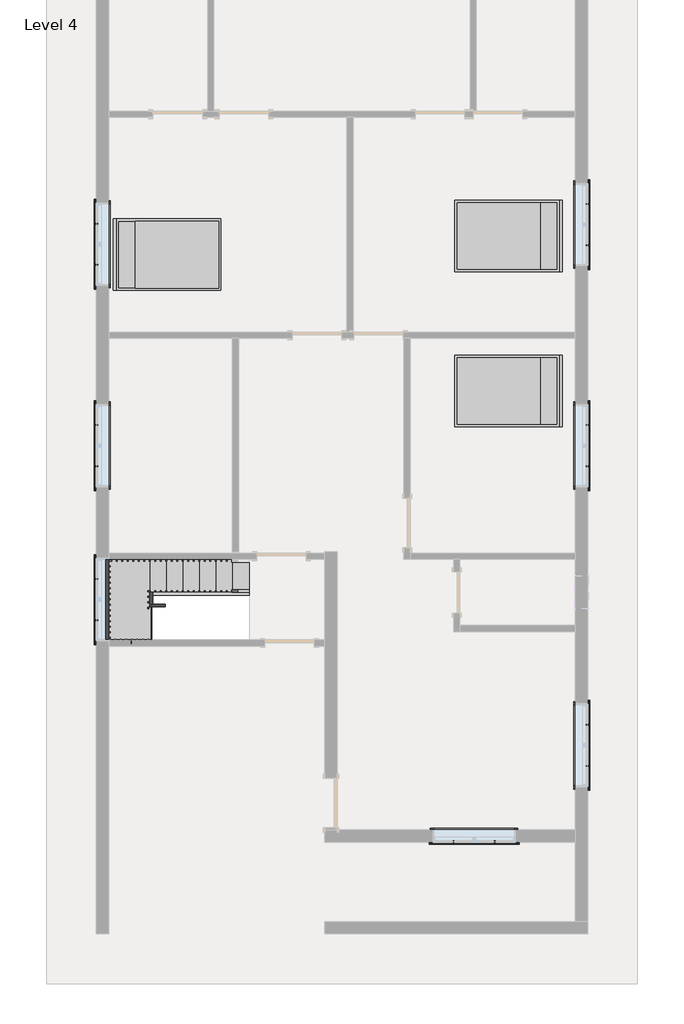
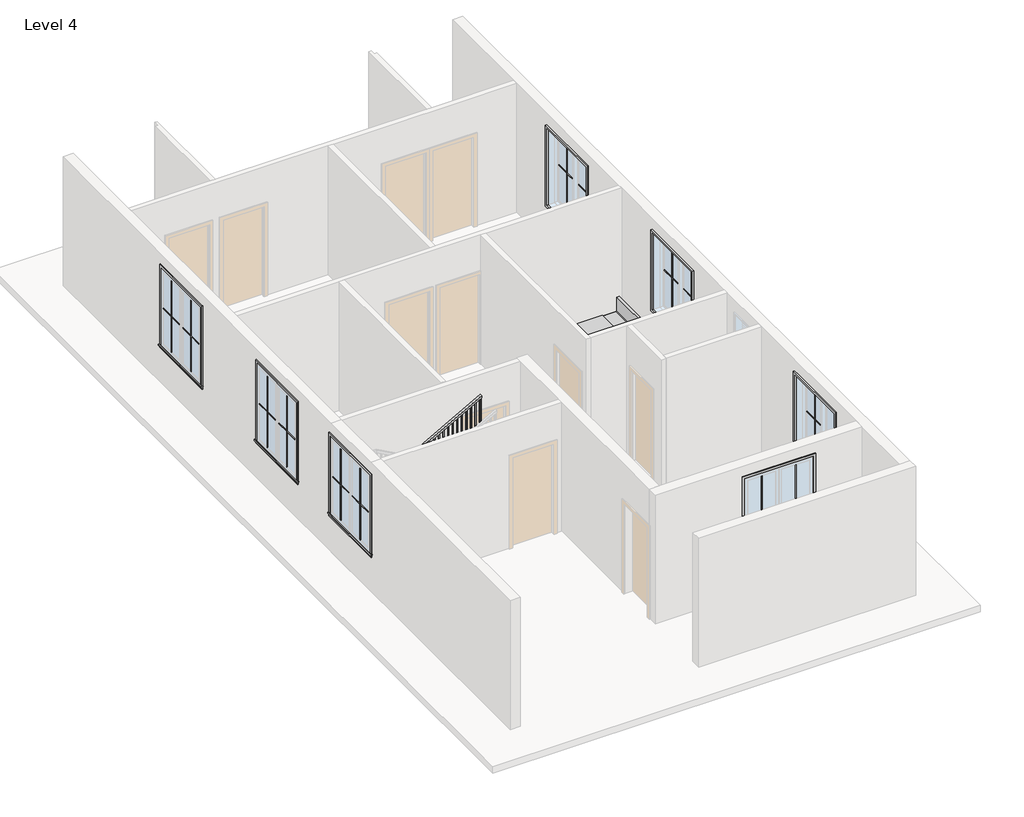
# One storey, part 3 of 3: 28 proxies, 6 members, 3 furniture elements, 1 railing, 1 stair flight.
"""IFC4 building model written with IfcOpenShell, lengths in millimetres."""

from ifc_helpers import new_model, si_unit, frame, origin, place, context, project, spatial, polyline, outline, extrude, faceted_brep, transform, mapped, element, save
from components import muntin_pattern_2x2_muntin_pattern_2x2_f6a80940, muntin_pattern_2x2_muntin_pattern_2x2_09b00a1c, trim_window_exterior_flat_with_sill_698ed857, trim_window_interior_flat_picture_frame_92551a5e, bed_17739_bed_17739_15c61121, stair_flight_6f8696f7

model = new_model("IFC4")

# Units and contexts
model_context = context("Model", 3, world=origin())
ifc_project = project(units=[si_unit("LENGTHUNIT", "METRE", prefix="MILLI")], contexts=[model_context])

# Site, building, storey
site = spatial("IfcSite", under=ifc_project)
building = spatial("IfcBuilding", under=site)
storey = spatial("IfcBuildingStorey", under=building, Name="Level 4", Elevation=6400.8)

# Proxies
placement = place(None, origin())
muntin_pattern_2x2_muntin_pattern_2x2_shape = muntin_pattern_2x2_muntin_pattern_2x2_f6a80940(model_context)
element("IfcBuildingElementProxy", 1, Name="Muntin Pattern_2x2 : Muntin Pattern_2x2", ObjectType="Muntin Pattern_2x2 : Muntin Pattern_2x2", at=placement, inside=storey, context=model_context, shape_type="MappedRepresentation", body=[
    mapped(muntin_pattern_2x2_muntin_pattern_2x2_shape, transform((-5778.6870155, 3260.8309309, 7385.05), x_axis=(0.0, 1.0, 0.0), y_axis=(-1.0, 0.0, 0.0), z_axis=(0.0, 0.0, 1.0))),
])
element("IfcBuildingElementProxy", 2, Name="Muntin Pattern_2x2 : Muntin Pattern_2x2", ObjectType="Muntin Pattern_2x2 : Muntin Pattern_2x2", at=placement, inside=storey, context=model_context, shape_type="MappedRepresentation", body=[
    mapped(muntin_pattern_2x2_muntin_pattern_2x2_shape, transform((3270.0629845, 4381.6059309, 7385.05), x_axis=(0.0, -1.0, 0.0), y_axis=(1.0, 0.0, 0.0), z_axis=(0.0, 0.0, 1.0))),
])
element("IfcBuildingElementProxy", 3, Name="Muntin Pattern_2x2 : Muntin Pattern_2x2", ObjectType="Muntin Pattern_2x2 : Muntin Pattern_2x2", at=placement, inside=storey, context=model_context, shape_type="MappedRepresentation", body=[
    mapped(muntin_pattern_2x2_muntin_pattern_2x2_shape, transform((3270.0629845, 304.9059309, 7385.05), x_axis=(0.0, -1.0, 0.0), y_axis=(1.0, 0.0, 0.0), z_axis=(0.0, 0.0, 1.0))),
])
element("IfcBuildingElementProxy", 4, Name="Muntin Pattern_2x2 : Muntin Pattern_2x2", ObjectType="Muntin Pattern_2x2 : Muntin Pattern_2x2", at=placement, inside=storey, context=model_context, shape_type="MappedRepresentation", body=[
    mapped(muntin_pattern_2x2_muntin_pattern_2x2_shape, transform((3270.0629845, -5219.5940691, 7385.05), x_axis=(0.0, -1.0, 0.0), y_axis=(1.0, 0.0, 0.0), z_axis=(0.0, 0.0, 1.0))),
])
element("IfcBuildingElementProxy", 5, Name="Muntin Pattern_2x2 : Muntin Pattern_2x2", ObjectType="Muntin Pattern_2x2 : Muntin Pattern_2x2", at=placement, inside=storey, context=model_context, shape_type="MappedRepresentation", body=[
    mapped(muntin_pattern_2x2_muntin_pattern_2x2_shape, transform((1563.5004845, -7380.1815691, 7385.05), x_axis=(-1.0, 0.0, 0.0), y_axis=(0.0, -1.0, 0.0), z_axis=(0.0, 0.0, 1.0))),
])
element("IfcBuildingElementProxy", 6, Name="Muntin Pattern_2x2 : Muntin Pattern_2x2", ObjectType="Muntin Pattern_2x2 : Muntin Pattern_2x2", at=placement, inside=storey, context=model_context, shape_type="MappedRepresentation", body=[
    mapped(muntin_pattern_2x2_muntin_pattern_2x2_shape, transform((-5778.6870155, -3292.3690691, 7385.05), x_axis=(0.0, 1.0, 0.0), y_axis=(-1.0, 0.0, 0.0), z_axis=(0.0, 0.0, 1.0))),
])
element("IfcBuildingElementProxy", 7, Name="Muntin Pattern_2x2 : Muntin Pattern_2x2", ObjectType="Muntin Pattern_2x2 : Muntin Pattern_2x2", at=placement, inside=storey, context=model_context, shape_type="MappedRepresentation", body=[
    mapped(muntin_pattern_2x2_muntin_pattern_2x2_shape, transform((-5778.6870155, -453.9190691, 7385.05), x_axis=(0.0, 1.0, 0.0), y_axis=(-1.0, 0.0, 0.0), z_axis=(0.0, 0.0, 1.0))),
])
muntin_pattern_2x2_muntin_pattern_2x2_2_shape = muntin_pattern_2x2_muntin_pattern_2x2_09b00a1c(model_context)
element("IfcBuildingElementProxy", 8, Name="Muntin Pattern_2x2 : Muntin Pattern_2x2", ObjectType="Muntin Pattern_2x2 : Muntin Pattern_2x2", at=placement, inside=storey, context=model_context, shape_type="MappedRepresentation", body=[
    mapped(muntin_pattern_2x2_muntin_pattern_2x2_2_shape, transform((-5778.6870155, 4019.6559309, 7385.05), x_axis=(0.0, -1.0, 0.0), y_axis=(1.0, 0.0, 0.0), z_axis=(0.0, 0.0, 1.0))),
])
element("IfcBuildingElementProxy", 9, Name="Muntin Pattern_2x2 : Muntin Pattern_2x2", ObjectType="Muntin Pattern_2x2 : Muntin Pattern_2x2", at=placement, inside=storey, context=model_context, shape_type="MappedRepresentation", body=[
    mapped(muntin_pattern_2x2_muntin_pattern_2x2_2_shape, transform((3270.0629845, 3622.7809309, 7385.05), x_axis=(0.0, 1.0, 0.0), y_axis=(-1.0, 0.0, 0.0), z_axis=(0.0, 0.0, 1.0))),
])
element("IfcBuildingElementProxy", 10, Name="Muntin Pattern_2x2 : Muntin Pattern_2x2", ObjectType="Muntin Pattern_2x2 : Muntin Pattern_2x2", at=placement, inside=storey, context=model_context, shape_type="MappedRepresentation", body=[
    mapped(muntin_pattern_2x2_muntin_pattern_2x2_2_shape, transform((3270.0629845, -453.9190691, 7385.05), x_axis=(0.0, 1.0, 0.0), y_axis=(-1.0, 0.0, 0.0), z_axis=(0.0, 0.0, 1.0))),
])
element("IfcBuildingElementProxy", 11, Name="Muntin Pattern_2x2 : Muntin Pattern_2x2", ObjectType="Muntin Pattern_2x2 : Muntin Pattern_2x2", at=placement, inside=storey, context=model_context, shape_type="MappedRepresentation", body=[
    mapped(muntin_pattern_2x2_muntin_pattern_2x2_2_shape, transform((3270.0629845, -5978.4190691, 7385.05), x_axis=(0.0, 1.0, 0.0), y_axis=(-1.0, 0.0, 0.0), z_axis=(0.0, 0.0, 1.0))),
])
element("IfcBuildingElementProxy", 12, Name="Muntin Pattern_2x2 : Muntin Pattern_2x2", ObjectType="Muntin Pattern_2x2 : Muntin Pattern_2x2", at=placement, inside=storey, context=model_context, shape_type="MappedRepresentation", body=[
    mapped(muntin_pattern_2x2_muntin_pattern_2x2_2_shape, transform((804.6754845, -7380.1815691, 7385.05), x_axis=(1.0, 0.0, 0.0), y_axis=(0.0, 1.0, 0.0), z_axis=(0.0, 0.0, 1.0))),
])
element("IfcBuildingElementProxy", 13, Name="Muntin Pattern_2x2 : Muntin Pattern_2x2", ObjectType="Muntin Pattern_2x2 : Muntin Pattern_2x2", at=placement, inside=storey, context=model_context, shape_type="MappedRepresentation", body=[
    mapped(muntin_pattern_2x2_muntin_pattern_2x2_2_shape, transform((-5778.6870155, -2533.5440691, 7385.05), x_axis=(0.0, -1.0, 0.0), y_axis=(1.0, 0.0, 0.0), z_axis=(0.0, 0.0, 1.0))),
])
element("IfcBuildingElementProxy", 14, Name="Muntin Pattern_2x2 : Muntin Pattern_2x2", ObjectType="Muntin Pattern_2x2 : Muntin Pattern_2x2", at=placement, inside=storey, context=model_context, shape_type="MappedRepresentation", body=[
    mapped(muntin_pattern_2x2_muntin_pattern_2x2_2_shape, transform((-5778.6870155, 304.9059309, 7385.05), x_axis=(0.0, -1.0, 0.0), y_axis=(1.0, 0.0, 0.0), z_axis=(0.0, 0.0, 1.0))),
])
trim_window_exterior_flat_with_sill_shape = trim_window_exterior_flat_with_sill_698ed857(model_context)
element("IfcBuildingElementProxy", 15, Name="Trim-Window-Exterior-Flat : with Sill", ObjectType="Trim-Window-Exterior-Flat : with Sill", at=placement, inside=storey, context=model_context, shape_type="MappedRepresentation", body=[
    mapped(trim_window_exterior_flat_with_sill_shape, transform((-5788.2120155, 3640.2434309, 9144.0), x_axis=(0.0, -1.0, 0.0), y_axis=(0.0, 0.0, 1.0), z_axis=(-1.0, 0.0, 0.0))),
])
element("IfcBuildingElementProxy", 16, Name="Trim-Window-Exterior-Flat : with Sill", ObjectType="Trim-Window-Exterior-Flat : with Sill", at=placement, inside=storey, context=model_context, shape_type="MappedRepresentation", body=[
    mapped(trim_window_exterior_flat_with_sill_shape, transform((3279.5879845, 4002.1934309, 9144.0), x_axis=(0.0, 1.0, 0.0), y_axis=(0.0, 0.0, 1.0), z_axis=(1.0, 0.0, 0.0))),
])
element("IfcBuildingElementProxy", 17, Name="Trim-Window-Exterior-Flat : with Sill", ObjectType="Trim-Window-Exterior-Flat : with Sill", at=placement, inside=storey, context=model_context, shape_type="MappedRepresentation", body=[
    mapped(trim_window_exterior_flat_with_sill_shape, transform((3279.5879845, -74.5065691, 9144.0), x_axis=(0.0, 1.0, 0.0), y_axis=(0.0, 0.0, 1.0), z_axis=(1.0, 0.0, 0.0))),
])
element("IfcBuildingElementProxy", 18, Name="Trim-Window-Exterior-Flat : with Sill", ObjectType="Trim-Window-Exterior-Flat : with Sill", at=placement, inside=storey, context=model_context, shape_type="MappedRepresentation", body=[
    mapped(trim_window_exterior_flat_with_sill_shape, transform((3279.5879845, -5599.0065691, 9144.0), x_axis=(0.0, 1.0, 0.0), y_axis=(0.0, 0.0, 1.0), z_axis=(1.0, 0.0, 0.0))),
])
element("IfcBuildingElementProxy", 19, Name="Trim-Window-Exterior-Flat : with Sill", ObjectType="Trim-Window-Exterior-Flat : with Sill", at=placement, inside=storey, context=model_context, shape_type="MappedRepresentation", body=[
    mapped(trim_window_exterior_flat_with_sill_shape, transform((1184.0879845, -7389.7065691, 9144.0), x_axis=(1.0, 0.0, 0.0), y_axis=(0.0, 0.0, 1.0), z_axis=(0.0, -1.0, 0.0))),
])
element("IfcBuildingElementProxy", 20, Name="Trim-Window-Exterior-Flat : with Sill", ObjectType="Trim-Window-Exterior-Flat : with Sill", at=placement, inside=storey, context=model_context, shape_type="MappedRepresentation", body=[
    mapped(trim_window_exterior_flat_with_sill_shape, transform((-5788.2120155, -2912.9565691, 9144.0), x_axis=(0.0, -1.0, 0.0), y_axis=(0.0, 0.0, 1.0), z_axis=(-1.0, 0.0, 0.0))),
])
element("IfcBuildingElementProxy", 21, Name="Trim-Window-Exterior-Flat : with Sill", ObjectType="Trim-Window-Exterior-Flat : with Sill", at=placement, inside=storey, context=model_context, shape_type="MappedRepresentation", body=[
    mapped(trim_window_exterior_flat_with_sill_shape, transform((-5788.2120155, -74.5065691, 9144.0), x_axis=(0.0, -1.0, 0.0), y_axis=(0.0, 0.0, 1.0), z_axis=(-1.0, 0.0, 0.0))),
])
trim_window_interior_flat_picture_frame_shape = trim_window_interior_flat_picture_frame_92551a5e(model_context)
element("IfcBuildingElementProxy", 22, Name="Trim-Window-Interior-Flat : Picture Frame", ObjectType="Trim-Window-Interior-Flat : Picture Frame", at=placement, inside=storey, context=model_context, shape_type="MappedRepresentation", body=[
    mapped(trim_window_interior_flat_picture_frame_shape, transform((-5559.6120155, 3640.2434309, 9144.0), x_axis=(0.0, 1.0, 0.0), y_axis=(0.0, 0.0, 1.0), z_axis=(1.0, 0.0, 0.0))),
])
element("IfcBuildingElementProxy", 23, Name="Trim-Window-Interior-Flat : Picture Frame", ObjectType="Trim-Window-Interior-Flat : Picture Frame", at=placement, inside=storey, context=model_context, shape_type="MappedRepresentation", body=[
    mapped(trim_window_interior_flat_picture_frame_shape, transform((3050.9879845, 4002.1934309, 9144.0), x_axis=(0.0, -1.0, 0.0), y_axis=(0.0, 0.0, 1.0), z_axis=(-1.0, 0.0, 0.0))),
])
element("IfcBuildingElementProxy", 24, Name="Trim-Window-Interior-Flat : Picture Frame", ObjectType="Trim-Window-Interior-Flat : Picture Frame", at=placement, inside=storey, context=model_context, shape_type="MappedRepresentation", body=[
    mapped(trim_window_interior_flat_picture_frame_shape, transform((3050.9879845, -74.5065691, 9144.0), x_axis=(0.0, -1.0, 0.0), y_axis=(0.0, 0.0, 1.0), z_axis=(-1.0, 0.0, 0.0))),
])
element("IfcBuildingElementProxy", 25, Name="Trim-Window-Interior-Flat : Picture Frame", ObjectType="Trim-Window-Interior-Flat : Picture Frame", at=placement, inside=storey, context=model_context, shape_type="MappedRepresentation", body=[
    mapped(trim_window_interior_flat_picture_frame_shape, transform((3050.9879845, -5599.0065691, 9144.0), x_axis=(0.0, -1.0, 0.0), y_axis=(0.0, 0.0, 1.0), z_axis=(-1.0, 0.0, 0.0))),
])
element("IfcBuildingElementProxy", 26, Name="Trim-Window-Interior-Flat : Picture Frame", ObjectType="Trim-Window-Interior-Flat : Picture Frame", at=placement, inside=storey, context=model_context, shape_type="MappedRepresentation", body=[
    mapped(trim_window_interior_flat_picture_frame_shape, transform((1184.0879845, -7161.1065691, 9144.0), x_axis=(-1.0, 0.0, 0.0), y_axis=(0.0, 0.0, 1.0), z_axis=(0.0, 1.0, 0.0))),
])
element("IfcBuildingElementProxy", 27, Name="Trim-Window-Interior-Flat : Picture Frame", ObjectType="Trim-Window-Interior-Flat : Picture Frame", at=placement, inside=storey, context=model_context, shape_type="MappedRepresentation", body=[
    mapped(trim_window_interior_flat_picture_frame_shape, transform((-5559.6120155, -2912.9565691, 9144.0), x_axis=(0.0, 1.0, 0.0), y_axis=(0.0, 0.0, 1.0), z_axis=(1.0, 0.0, 0.0))),
])
element("IfcBuildingElementProxy", 28, Name="Trim-Window-Interior-Flat : Picture Frame", ObjectType="Trim-Window-Interior-Flat : Picture Frame", at=placement, inside=storey, context=model_context, shape_type="MappedRepresentation", body=[
    mapped(trim_window_interior_flat_picture_frame_shape, transform((-5559.6120155, -74.5065691, 9144.0), x_axis=(0.0, 1.0, 0.0), y_axis=(0.0, 0.0, 1.0), z_axis=(1.0, 0.0, 0.0))),
])

# Furniture
bed_17739_bed_17739_shape = bed_17739_bed_17739_15c61121(model_context)
element("IfcFurniture", 29, ObjectType="Bed_17739 : Bed_17739", at=placement, inside=storey, context=model_context, shape_type="MappedRepresentation", body=[
    mapped(bed_17739_bed_17739_shape, transform((-4454.7120155, 3449.7434309, 6400.8), x_axis=(0.0, 1.0, 0.0), y_axis=(-1.0, 0.0, 0.0), z_axis=(0.0, 0.0, 1.0))),
])
element("IfcFurniture", 30, ObjectType="Bed_17739 : Bed_17739", at=placement, inside=storey, context=model_context, shape_type="MappedRepresentation", body=[
    mapped(bed_17739_bed_17739_shape, transform((1793.6879845, 3792.6434309, 6400.8), x_axis=(0.0, -1.0, 0.0), y_axis=(1.0, 0.0, 0.0), z_axis=(0.0, 0.0, 1.0))),
])
element("IfcFurniture", 31, ObjectType="Bed_17739 : Bed_17739", at=placement, inside=storey, context=model_context, shape_type="MappedRepresentation", body=[
    mapped(bed_17739_bed_17739_shape, transform((1793.6879845, 935.1434309, 6400.8), x_axis=(0.0, -1.0, 0.0), y_axis=(1.0, 0.0, 0.0), z_axis=(0.0, 0.0, 1.0))),
])

# Members
element("IfcMember", 32, ObjectType="Stringer - 2\" Width", at=placement, inside=storey, context=model_context, shape_type="SweptSolid", body=[
    extrude(outline(polyline([(6400.8, -2968.8120155), (6608.3983948, -2968.8120155), (7596.1761726, -4746.8120155), (7247.4974984, -4746.8120155), (6400.8, -3222.7565183), (6400.8, -2968.8120155)])), frame((0.0, -2830.4065691, 0.0), z_axis=(0.0, 1.0, 0.0), x_axis=(0.0, 0.0, 1.0)), (0.0, 0.0, 1.0), 50.8),
])
element("IfcMember", 33, ObjectType="Stringer - 2\" Width", at=placement, inside=storey, context=model_context, shape_type="SweptSolid", body=[
    extrude(outline(polyline([(-4797.6120155, -2779.6065691), (-4746.8120155, -2779.6065691), (-4746.8120155, -2995.5065691), (-4797.6120155, -2995.5065691), (-4797.6120155, -2779.6065691)])), frame((0.0, 0.0, 7357.5333333), z_axis=(0.0, 0.0, 1.0), x_axis=(1.0, 0.0, 0.0)), (0.0, 0.0, 1.0), 304.8),
])
element("IfcMember", 34, ObjectType="Stringer - 2\" Width", at=placement, inside=storey, context=model_context, shape_type="SweptSolid", body=[
    extrude(outline(polyline([(7793.7317281, -4797.6120155), (7445.053054, -4797.6120155), (8461.053054, -2968.8120155), (8809.7317281, -2968.8120155), (7793.7317281, -4797.6120155)])), frame((0.0, -3046.3065691, 0.0), z_axis=(0.0, 1.0, 0.0), x_axis=(0.0, 0.0, 1.0)), (0.0, 0.0, 1.0), 50.8),
])
element("IfcMember", 35, ObjectType="Stringer - 2\" Width", at=placement, inside=storey, context=model_context, shape_type="SweptSolid", body=[
    extrude(outline(polyline([(6400.8, -2968.8120155), (6608.3983948, -2968.8120155), (7662.3333333, -4865.8949049), (7662.3333333, -5493.5165183), (6400.8, -3222.7565183), (6400.8, -2968.8120155)])), frame((0.0, -2170.0065691, 0.0), z_axis=(0.0, 1.0, 0.0), x_axis=(0.0, 0.0, 1.0)), (0.0, 0.0, 1.0), 50.8),
])
element("IfcMember", 36, ObjectType="Stringer - 2\" Width", at=placement, inside=storey, context=model_context, shape_type="SweptSolid", body=[
    extrude(outline(polyline([(-5610.4120155, -2119.2065691), (-5559.6120155, -2119.2065691), (-5559.6120155, -3674.9565691), (-5610.4120155, -3674.9565691), (-5610.4120155, -2119.2065691)])), frame((0.0, 0.0, 7357.5333333), z_axis=(0.0, 0.0, 1.0), x_axis=(1.0, 0.0, 0.0)), (0.0, 0.0, 1.0), 304.8),
])
element("IfcMember", 37, ObjectType="Stringer - 2\" Width", at=placement, inside=storey, context=model_context, shape_type="SweptSolid", body=[
    extrude(outline(polyline([(7357.5333333, -4955.1475127), (8461.053054, -2968.8120155), (8809.7317281, -2968.8120155), (7357.5333333, -5582.7691261), (7357.5333333, -4955.1475127)])), frame((0.0, -3725.7565691, 0.0), z_axis=(0.0, 1.0, 0.0), x_axis=(0.0, 0.0, 1.0)), (0.0, 0.0, 1.0), 50.8),
])

# Railing
element("IfcRailing", 38, ObjectType="Handrail - Rectangular", at=placement, inside=storey, context=model_context, shape_type="SolidModel", body=[
    faceted_brep([(-2968.8120155, -2779.6065691, 7484.5333333), (-2968.8120155, -2779.6065691, 7426.420221), (-2968.8120155, -2728.8065691, 7426.420221), (-2968.8120155, -2728.8065691, 7484.5333333), (-4721.4120155, -2779.6065691, 8458.2), (-4772.2120155, -2779.6065691, 8428.3091099), (-4772.2120155, -2728.8065691, 8428.3091099), (-4721.4120155, -2728.8065691, 8458.2), (-4721.4120155, -2779.6065691, 8500.5333333), (-4772.2120155, -2779.6065691, 8449.7333333), (-4772.2120155, -2728.8065691, 8449.7333333), (-4721.4120155, -2728.8065691, 8500.5333333), (-4797.6120155, -2779.6065691, 8500.5333333), (-4797.6120155, -2779.6065691, 8449.7333333), (-4848.4120155, -2728.8065691, 8449.7333333), (-4848.4120155, -2728.8065691, 8500.5333333), (-4797.6120155, -2855.8065691, 8500.5333333), (-4797.6120155, -2855.8065691, 8449.7333333), (-4848.4120155, -2855.8065691, 8449.7333333), (-4848.4120155, -2855.8065691, 8500.5333333), (-4797.6120155, -2970.1065691, 8500.5333333), (-4797.6120155, -3020.9065691, 8449.7333333), (-4848.4120155, -3020.9065691, 8449.7333333), (-4848.4120155, -2970.1065691, 8500.5333333), (-4797.6120155, -2970.1065691, 8712.2), (-4797.6120155, -3020.9065691, 8661.4), (-4848.4120155, -3020.9065691, 8661.4), (-4848.4120155, -2970.1065691, 8712.2), (-4797.6120155, -3046.3065691, 8712.2), (-4797.6120155, -3046.3065691, 8661.4), (-4848.4120155, -3097.1065691, 8661.4), (-4848.4120155, -3097.1065691, 8712.2), (-4721.4120155, -3046.3065691, 8712.2), (-4708.2484132, -3046.3065691, 8661.4), (-4708.2484132, -3097.1065691, 8661.4), (-4721.4120155, -3097.1065691, 8712.2), (-2968.8120155, -3046.3065691, 9685.8666667), (-2968.8120155, -3097.1065691, 9685.8666667), (-2968.8120155, -3097.1065691, 9627.7535543), (-2968.8120155, -3046.3065691, 9627.7535543)], [[[0, 1, 2, 3]], [[1, 0, 4, 5]], [[2, 1, 5, 6]], [[3, 2, 6, 7]], [[0, 3, 7, 4]], [[5, 4, 8, 9]], [[6, 5, 9, 10]], [[7, 6, 10, 11]], [[4, 7, 11, 8]], [[9, 8, 12, 13]], [[10, 9, 13, 14]], [[11, 10, 14, 15]], [[8, 11, 15, 12]], [[13, 12, 16, 17]], [[14, 13, 17, 18]], [[15, 14, 18, 19]], [[12, 15, 19, 16]], [[17, 16, 20, 21]], [[18, 17, 21, 22]], [[19, 18, 22, 23]], [[16, 19, 23, 20]], [[21, 20, 24, 25]], [[22, 21, 25, 26]], [[23, 22, 26, 27]], [[20, 23, 27, 24]], [[25, 24, 28, 29]], [[26, 25, 29, 30]], [[27, 26, 30, 31]], [[24, 27, 31, 28]], [[29, 28, 32, 33]], [[30, 29, 33, 34]], [[31, 30, 34, 35]], [[28, 31, 35, 32]], [[36, 37, 38, 39]], [[33, 32, 36, 39]], [[34, 33, 39, 38]], [[35, 34, 38, 37]], [[32, 35, 37, 36]]]),
    extrude(outline(polyline([(9608.3507765, -3003.7370155), (8602.1333333, -3003.7370155), (8602.1333333, -2984.6870155), (9618.9341099, -2984.6870155), (9608.3507765, -3003.7370155)])), frame((0.0, -3081.2315691, 0.0), z_axis=(0.0, 1.0, 0.0), x_axis=(0.0, 0.0, 1.0)), (0.0, 0.0, 1.0), 19.05),
    extrude(outline(polyline([(9551.9063321, -3105.3370155), (8602.1333333, -3105.3370155), (8602.1333333, -3086.2870155), (9562.4896654, -3086.2870155), (9551.9063321, -3105.3370155)])), frame((0.0, -3081.2315691, 0.0), z_axis=(0.0, 1.0, 0.0), x_axis=(0.0, 0.0, 1.0)), (0.0, 0.0, 1.0), 19.05),
    extrude(outline(polyline([(9495.4618876, -3206.9370155), (8602.1333333, -3206.9370155), (8602.1333333, -3187.8870155), (9506.045221, -3187.8870155), (9495.4618876, -3206.9370155)])), frame((0.0, -3081.2315691, 0.0), z_axis=(0.0, 1.0, 0.0), x_axis=(0.0, 0.0, 1.0)), (0.0, 0.0, 1.0), 19.05),
    extrude(outline(polyline([(9439.0174432, -3308.5370155), (8432.8, -3308.5370155), (8432.8, -3289.4870155), (9449.6007765, -3289.4870155), (9439.0174432, -3308.5370155)])), frame((0.0, -3081.2315691, 0.0), z_axis=(0.0, 1.0, 0.0), x_axis=(0.0, 0.0, 1.0)), (0.0, 0.0, 1.0), 19.05),
    extrude(outline(polyline([(9382.5729988, -3410.1370155), (8432.8, -3410.1370155), (8432.8, -3391.0870155), (9393.1563321, -3391.0870155), (9382.5729988, -3410.1370155)])), frame((0.0, -3081.2315691, 0.0), z_axis=(0.0, 1.0, 0.0), x_axis=(0.0, 0.0, 1.0)), (0.0, 0.0, 1.0), 19.05),
    extrude(outline(polyline([(9326.1285543, -3511.7370155), (8432.8, -3511.7370155), (8432.8, -3492.6870155), (9336.7118876, -3492.6870155), (9326.1285543, -3511.7370155)])), frame((0.0, -3081.2315691, 0.0), z_axis=(0.0, 1.0, 0.0), x_axis=(0.0, 0.0, 1.0)), (0.0, 0.0, 1.0), 19.05),
    extrude(outline(polyline([(9269.6841099, -3613.3370155), (8263.4666667, -3613.3370155), (8263.4666667, -3594.2870155), (9280.2674432, -3594.2870155), (9269.6841099, -3613.3370155)])), frame((0.0, -3081.2315691, 0.0), z_axis=(0.0, 1.0, 0.0), x_axis=(0.0, 0.0, 1.0)), (0.0, 0.0, 1.0), 19.05),
    extrude(outline(polyline([(9213.2396654, -3714.9370155), (8263.4666667, -3714.9370155), (8263.4666667, -3695.8870155), (9223.8229988, -3695.8870155), (9213.2396654, -3714.9370155)])), frame((0.0, -3081.2315691, 0.0), z_axis=(0.0, 1.0, 0.0), x_axis=(0.0, 0.0, 1.0)), (0.0, 0.0, 1.0), 19.05),
    extrude(outline(polyline([(9156.795221, -3816.5370155), (8263.4666667, -3816.5370155), (8263.4666667, -3797.4870155), (9167.3785543, -3797.4870155), (9156.795221, -3816.5370155)])), frame((0.0, -3081.2315691, 0.0), z_axis=(0.0, 1.0, 0.0), x_axis=(0.0, 0.0, 1.0)), (0.0, 0.0, 1.0), 19.05),
    extrude(outline(polyline([(9100.3507765, -3918.1370155), (8094.1333333, -3918.1370155), (8094.1333333, -3899.0870155), (9110.9341099, -3899.0870155), (9100.3507765, -3918.1370155)])), frame((0.0, -3081.2315691, 0.0), z_axis=(0.0, 1.0, 0.0), x_axis=(0.0, 0.0, 1.0)), (0.0, 0.0, 1.0), 19.05),
    extrude(outline(polyline([(9043.9063321, -4019.7370155), (8094.1333333, -4019.7370155), (8094.1333333, -4000.6870155), (9054.4896654, -4000.6870155), (9043.9063321, -4019.7370155)])), frame((0.0, -3081.2315691, 0.0), z_axis=(0.0, 1.0, 0.0), x_axis=(0.0, 0.0, 1.0)), (0.0, 0.0, 1.0), 19.05),
    extrude(outline(polyline([(8987.4618876, -4121.3370155), (8094.1333333, -4121.3370155), (8094.1333333, -4102.2870155), (8998.045221, -4102.2870155), (8987.4618876, -4121.3370155)])), frame((0.0, -3081.2315691, 0.0), z_axis=(0.0, 1.0, 0.0), x_axis=(0.0, 0.0, 1.0)), (0.0, 0.0, 1.0), 19.05),
    extrude(outline(polyline([(8931.0174432, -4222.9370155), (7924.8, -4222.9370155), (7924.8, -4203.8870155), (8941.6007765, -4203.8870155), (8931.0174432, -4222.9370155)])), frame((0.0, -3081.2315691, 0.0), z_axis=(0.0, 1.0, 0.0), x_axis=(0.0, 0.0, 1.0)), (0.0, 0.0, 1.0), 19.05),
    extrude(outline(polyline([(8874.5729988, -4324.5370155), (7924.8, -4324.5370155), (7924.8, -4305.4870155), (8885.1563321, -4305.4870155), (8874.5729988, -4324.5370155)])), frame((0.0, -3081.2315691, 0.0), z_axis=(0.0, 1.0, 0.0), x_axis=(0.0, 0.0, 1.0)), (0.0, 0.0, 1.0), 19.05),
    extrude(outline(polyline([(8818.1285543, -4426.1370155), (7924.8, -4426.1370155), (7924.8, -4407.0870155), (8828.7118876, -4407.0870155), (8818.1285543, -4426.1370155)])), frame((0.0, -3081.2315691, 0.0), z_axis=(0.0, 1.0, 0.0), x_axis=(0.0, 0.0, 1.0)), (0.0, 0.0, 1.0), 19.05),
    extrude(outline(polyline([(8761.6841099, -4527.7370155), (7755.4666667, -4527.7370155), (7755.4666667, -4508.6870155), (8772.2674432, -4508.6870155), (8761.6841099, -4527.7370155)])), frame((0.0, -3081.2315691, 0.0), z_axis=(0.0, 1.0, 0.0), x_axis=(0.0, 0.0, 1.0)), (0.0, 0.0, 1.0), 19.05),
    extrude(outline(polyline([(8705.2396654, -4629.3370155), (7755.4666667, -4629.3370155), (7755.4666667, -4610.2870155), (8715.8229988, -4610.2870155), (8705.2396654, -4629.3370155)])), frame((0.0, -3081.2315691, 0.0), z_axis=(0.0, 1.0, 0.0), x_axis=(0.0, 0.0, 1.0)), (0.0, 0.0, 1.0), 19.05),
    extrude(outline(polyline([(8648.795221, -4730.9370155), (7755.4666667, -4730.9370155), (7755.4666667, -4711.8870155), (8659.3785543, -4711.8870155), (8648.795221, -4730.9370155)])), frame((0.0, -3081.2315691, 0.0), z_axis=(0.0, 1.0, 0.0), x_axis=(0.0, 0.0, 1.0)), (0.0, 0.0, 1.0), 19.05),
    extrude(outline(polyline([(-4813.4870155, -3049.4815691), (-4813.4870155, -3068.5315691), (-4832.5370155, -3068.5315691), (-4832.5370155, -3049.4815691), (-4813.4870155, -3049.4815691)])), frame((0.0, 0.0, 7586.1333333), z_axis=(0.0, 0.0, 1.0), x_axis=(1.0, 0.0, 0.0)), (0.0, 0.0, 1.0), 1075.2666667),
    extrude(outline(polyline([(-4813.4870155, -2947.8815691), (-4813.4870155, -2966.9315691), (-4832.5370155, -2966.9315691), (-4832.5370155, -2947.8815691), (-4813.4870155, -2947.8815691)])), frame((0.0, 0.0, 7586.1333333), z_axis=(0.0, 0.0, 1.0), x_axis=(1.0, 0.0, 0.0)), (0.0, 0.0, 1.0), 863.6),
    extrude(outline(polyline([(-4813.4870155, -2846.2815691), (-4813.4870155, -2865.3315691), (-4832.5370155, -2865.3315691), (-4832.5370155, -2846.2815691), (-4813.4870155, -2846.2815691)])), frame((0.0, 0.0, 7586.1333333), z_axis=(0.0, 0.0, 1.0), x_axis=(1.0, 0.0, 0.0)), (0.0, 0.0, 1.0), 863.6),
    extrude(outline(polyline([(-4788.0870155, -2763.7315691), (-4807.1370155, -2763.7315691), (-4807.1370155, -2744.6815691), (-4788.0870155, -2744.6815691), (-4788.0870155, -2763.7315691)])), frame((0.0, 0.0, 7586.1333333), z_axis=(0.0, 0.0, 1.0), x_axis=(1.0, 0.0, 0.0)), (0.0, 0.0, 1.0), 863.6),
    extrude(outline(polyline([(8391.2674432, -4705.5370155), (7416.8, -4705.5370155), (7416.8, -4686.4870155), (8380.6841099, -4686.4870155), (8391.2674432, -4705.5370155)])), frame((0.0, -2763.7315691, 0.0), z_axis=(0.0, 1.0, 0.0), x_axis=(0.0, 0.0, 1.0)), (0.0, 0.0, 1.0), 19.05),
    extrude(outline(polyline([(8334.8229988, -4603.9370155), (7416.8, -4603.9370155), (7416.8, -4584.8870155), (8324.2396654, -4584.8870155), (8334.8229988, -4603.9370155)])), frame((0.0, -2763.7315691, 0.0), z_axis=(0.0, 1.0, 0.0), x_axis=(0.0, 0.0, 1.0)), (0.0, 0.0, 1.0), 19.05),
    extrude(outline(polyline([(8278.3785543, -4502.3370155), (7416.8, -4502.3370155), (7416.8, -4483.2870155), (8267.795221, -4483.2870155), (8278.3785543, -4502.3370155)])), frame((0.0, -2763.7315691, 0.0), z_axis=(0.0, 1.0, 0.0), x_axis=(0.0, 0.0, 1.0)), (0.0, 0.0, 1.0), 19.05),
    extrude(outline(polyline([(8221.9341099, -4400.7370155), (7247.4666667, -4400.7370155), (7247.4666667, -4381.6870155), (8211.3507765, -4381.6870155), (8221.9341099, -4400.7370155)])), frame((0.0, -2763.7315691, 0.0), z_axis=(0.0, 1.0, 0.0), x_axis=(0.0, 0.0, 1.0)), (0.0, 0.0, 1.0), 19.05),
    extrude(outline(polyline([(8165.4896654, -4299.1370155), (7247.4666667, -4299.1370155), (7247.4666667, -4280.0870155), (8154.9063321, -4280.0870155), (8165.4896654, -4299.1370155)])), frame((0.0, -2763.7315691, 0.0), z_axis=(0.0, 1.0, 0.0), x_axis=(0.0, 0.0, 1.0)), (0.0, 0.0, 1.0), 19.05),
    extrude(outline(polyline([(8109.045221, -4197.5370155), (7247.4666667, -4197.5370155), (7247.4666667, -4178.4870155), (8098.4618876, -4178.4870155), (8109.045221, -4197.5370155)])), frame((0.0, -2763.7315691, 0.0), z_axis=(0.0, 1.0, 0.0), x_axis=(0.0, 0.0, 1.0)), (0.0, 0.0, 1.0), 19.05),
    extrude(outline(polyline([(8052.6007765, -4095.9370155), (7078.1333333, -4095.9370155), (7078.1333333, -4076.8870155), (8042.0174432, -4076.8870155), (8052.6007765, -4095.9370155)])), frame((0.0, -2763.7315691, 0.0), z_axis=(0.0, 1.0, 0.0), x_axis=(0.0, 0.0, 1.0)), (0.0, 0.0, 1.0), 19.05),
    extrude(outline(polyline([(7996.1563321, -3994.3370155), (7078.1333333, -3994.3370155), (7078.1333333, -3975.2870155), (7985.5729988, -3975.2870155), (7996.1563321, -3994.3370155)])), frame((0.0, -2763.7315691, 0.0), z_axis=(0.0, 1.0, 0.0), x_axis=(0.0, 0.0, 1.0)), (0.0, 0.0, 1.0), 19.05),
    extrude(outline(polyline([(7939.7118876, -3892.7370155), (7078.1333333, -3892.7370155), (7078.1333333, -3873.6870155), (7929.1285543, -3873.6870155), (7939.7118876, -3892.7370155)])), frame((0.0, -2763.7315691, 0.0), z_axis=(0.0, 1.0, 0.0), x_axis=(0.0, 0.0, 1.0)), (0.0, 0.0, 1.0), 19.05),
    extrude(outline(polyline([(7883.2674432, -3791.1370155), (6908.8, -3791.1370155), (6908.8, -3772.0870155), (7872.6841099, -3772.0870155), (7883.2674432, -3791.1370155)])), frame((0.0, -2763.7315691, 0.0), z_axis=(0.0, 1.0, 0.0), x_axis=(0.0, 0.0, 1.0)), (0.0, 0.0, 1.0), 19.05),
    extrude(outline(polyline([(7826.8229988, -3689.5370155), (6908.8, -3689.5370155), (6908.8, -3670.4870155), (7816.2396654, -3670.4870155), (7826.8229988, -3689.5370155)])), frame((0.0, -2763.7315691, 0.0), z_axis=(0.0, 1.0, 0.0), x_axis=(0.0, 0.0, 1.0)), (0.0, 0.0, 1.0), 19.05),
    extrude(outline(polyline([(7770.3785543, -3587.9370155), (6908.8, -3587.9370155), (6908.8, -3568.8870155), (7759.795221, -3568.8870155), (7770.3785543, -3587.9370155)])), frame((0.0, -2763.7315691, 0.0), z_axis=(0.0, 1.0, 0.0), x_axis=(0.0, 0.0, 1.0)), (0.0, 0.0, 1.0), 19.05),
    extrude(outline(polyline([(7713.9341099, -3486.3370155), (6739.4666667, -3486.3370155), (6739.4666667, -3467.2870155), (7703.3507765, -3467.2870155), (7713.9341099, -3486.3370155)])), frame((0.0, -2763.7315691, 0.0), z_axis=(0.0, 1.0, 0.0), x_axis=(0.0, 0.0, 1.0)), (0.0, 0.0, 1.0), 19.05),
    extrude(outline(polyline([(7657.4896654, -3384.7370155), (6739.4666667, -3384.7370155), (6739.4666667, -3365.6870155), (7646.9063321, -3365.6870155), (7657.4896654, -3384.7370155)])), frame((0.0, -2763.7315691, 0.0), z_axis=(0.0, 1.0, 0.0), x_axis=(0.0, 0.0, 1.0)), (0.0, 0.0, 1.0), 19.05),
    extrude(outline(polyline([(7601.045221, -3283.1370155), (6739.4666667, -3283.1370155), (6739.4666667, -3264.0870155), (7590.4618876, -3264.0870155), (7601.045221, -3283.1370155)])), frame((0.0, -2763.7315691, 0.0), z_axis=(0.0, 1.0, 0.0), x_axis=(0.0, 0.0, 1.0)), (0.0, 0.0, 1.0), 19.05),
    extrude(outline(polyline([(7544.6007765, -3181.5370155), (6570.1333333, -3181.5370155), (6570.1333333, -3162.4870155), (7534.0174432, -3162.4870155), (7544.6007765, -3181.5370155)])), frame((0.0, -2763.7315691, 0.0), z_axis=(0.0, 1.0, 0.0), x_axis=(0.0, 0.0, 1.0)), (0.0, 0.0, 1.0), 19.05),
    extrude(outline(polyline([(7488.1563321, -3079.9370155), (6570.1333333, -3079.9370155), (6570.1333333, -3060.8870155), (7477.5729988, -3060.8870155), (7488.1563321, -3079.9370155)])), frame((0.0, -2763.7315691, 0.0), z_axis=(0.0, 1.0, 0.0), x_axis=(0.0, 0.0, 1.0)), (0.0, 0.0, 1.0), 19.05),
    extrude(outline(polyline([(-4813.4870155, -3062.1815691), (-4813.4870155, -3081.2315691), (-4832.5370155, -3081.2315691), (-4832.5370155, -3062.1815691), (-4813.4870155, -3062.1815691)])), frame((0.0, 0.0, 7586.1333333), z_axis=(0.0, 0.0, 1.0), x_axis=(1.0, 0.0, 0.0)), (0.0, 0.0, 1.0), 1075.2666667),
    extrude(outline(polyline([(-4813.4870155, -2763.7315691), (-4832.5370155, -2763.7315691), (-4832.5370155, -2744.6815691), (-4813.4870155, -2744.6815691), (-4813.4870155, -2763.7315691)])), frame((0.0, 0.0, 7586.1333333), z_axis=(0.0, 0.0, 1.0), x_axis=(1.0, 0.0, 0.0)), (0.0, 0.0, 1.0), 863.6),
    extrude(outline(polyline([(9617.170221, -2987.8620155), (8602.1333333, -2987.8620155), (8602.1333333, -2968.8120155), (9627.7535543, -2968.8120155), (9617.170221, -2987.8620155)])), frame((0.0, -3081.2315691, 0.0), z_axis=(0.0, 1.0, 0.0), x_axis=(0.0, 0.0, 1.0)), (0.0, 0.0, 1.0), 19.05),
    extrude(outline(polyline([(7437.0035543, -2987.8620155), (6570.1333333, -2987.8620155), (6570.1333333, -2968.8120155), (7426.420221, -2968.8120155), (7437.0035543, -2987.8620155)])), frame((0.0, -2763.7315691, 0.0), z_axis=(0.0, 1.0, 0.0), x_axis=(0.0, 0.0, 1.0)), (0.0, 0.0, 1.0), 19.05),
])

# Stair flight
stair_flight_shape = stair_flight_6f8696f7(model_context)
element("IfcStairFlight", 39, ObjectType="2\" Tread 1\" Nosing 1/4\" Riser", at=placement, inside=storey, context=model_context, shape_type="MappedRepresentation", body=[
    mapped(stair_flight_shape, transform((0.0, 0.0, 0.0), x_axis=(1.0, 0.0, 0.0), y_axis=(0.0, 1.0, 0.0), z_axis=(0.0, 0.0, 1.0))),
])

save(model, "model.ifc")

# Revit data of these elements
# Type "Muntin Pattern_2x2 : Muntin Pattern_2x2"
#   Width [instance default] = 4' - 0"
#   Thickness = 0' - 0 1/2"
#   Height [instance default] = 4' - 0"
#   Distance = 0' - 0 3/4"
#   Interior Material [instance default] = none
#   Exterior Material [instance default] = none
#   Default Elevation = 0
# Type "Trim-Window-Exterior-Flat : with Sill"
#   Trim Width = 0' - 2 1/4"
#   Trim Thickness_Picture Frame = 0' - 1 1/4"
#   Trim Thickness_with Sill = 0' - 0 3/4"
#   Sill Thickness = 0' - 1 1/4"
#   Opening Width [instance default] = 2' - 0"
#   Opening Height [instance default] = 3' - 0"
#   Default Elevation = 4' - 0"
#   Sill = yes
#   Picture Frame = no
#   Trim Material [instance default] = none
# Type "Trim-Window-Interior-Flat : Picture Frame"
#   Trim Thickness_Picture Frame = 0' - 1 1/4"
#   Trim Width = 0' - 2 1/4"
#   Trim Thickness_with Sill = 0' - 0 3/4"
#   Sill Thickness = 0' - 1 1/4"
#   Opening Width [instance default] = 2' - 0"
#   Opening Height [instance default] = 3' - 0"
#   Default Elevation = 4' - 0"
#   Sill = no
#   Picture Frame = yes
#   Trim Material [instance default] = none
# Type "Bed_17739 : Bed_17739"
#   Default Elevation = 0
# Type "Handrail - Rectangular"
#   Assembly Code = "C2010400"
#   built-in parameter 1008612 = 0.0416667 (stored number, unit not read)
#   built-in parameter 1008611 = 0.0416667 (stored number, unit not read)
#   built-in parameter 1008609 = 0.333333 (stored number, unit not read)
#   built-in parameter 1008604 = 0.166667 (stored number, unit not read)
#   built-in parameter 1008603 = 0.166667 (stored number, unit not read)
#   Railing Height = 3' - 0"
#   built-in parameter 1008630 = 2
#   built-in parameter 1008610 = 2
#   built-in parameter 1008618 = Baluster - Square : 3/4"
# Elements 1, 2, 3, 4, 5, 6, 7, 8, 9, 10, 11, 12, 13, 14 (IfcBuildingElementProxy, "Muntin Pattern_2x2 : Muntin Pattern_2x2")
#   Width = 2' - 0 5/8"
#   Height = 5' - 6 1/2"
#   Interior Material = Wood - Stained
#   Exterior Material = Clad - White
#   Phase Created = New Construction
#   Materials on its faces: "Clad - White", "Wood - Stained"
# Elements 15, 16, 17, 18, 19, 20, 21 (IfcBuildingElementProxy, "Trim-Window-Exterior-Flat : with Sill")
#   Opening Width = 5' - 0"
#   Opening Height = 6' - 0"
#   Trim Material = Clad - White
#   Phase Created = New Construction
#   Materials on its faces: "Clad - White"
# Elements 22, 23, 24, 25, 26, 27, 28 (IfcBuildingElementProxy, "Trim-Window-Interior-Flat : Picture Frame")
#   Opening Width = 5' - 0"
#   Opening Height = 6' - 0"
#   Trim Material = Wood - Stained
#   Phase Created = New Construction
#   Materials on its faces: "Wood - Stained"
# Elements 29, 30, 31 (IfcFurniture, "Bed_17739 : Bed_17739")
#   Phase Created = New Construction
#   Materials on its faces: "legs", "sheets", "bed frame", "Blanket"
# Elements 32, 33, 34, 35, 36, 37 (IfcMember, "Stringer - 2\" Width")
#   Phase Created = New Construction
# Element 38 (IfcRailing, "Handrail - Rectangular")
#   Phase Created = New Construction
# Element 39 (IfcStairFlight, "2\" Tread 1\" Nosing 1/4\" Riser")
#   Phase Created = New Construction
# Materials
#   "Clad - White": class "Wood", colour RGB 242 242 238, transparency 0, Cost = 0
#   "Wood - Stained": class "Wood", colour RGB 224 178 126, transparency 0, Cost = 0
#   "legs": colour RGB 90 73 37, transparency 0, Cost = 0
#   "sheets": colour RGB 200 195 176, transparency 0, Cost = 0
#   "bed frame": colour RGB 90 73 37, transparency 0, Cost = 0
#   "Blanket": class "System", colour RGB 59 0 1, transparency 0, Cost = 0
